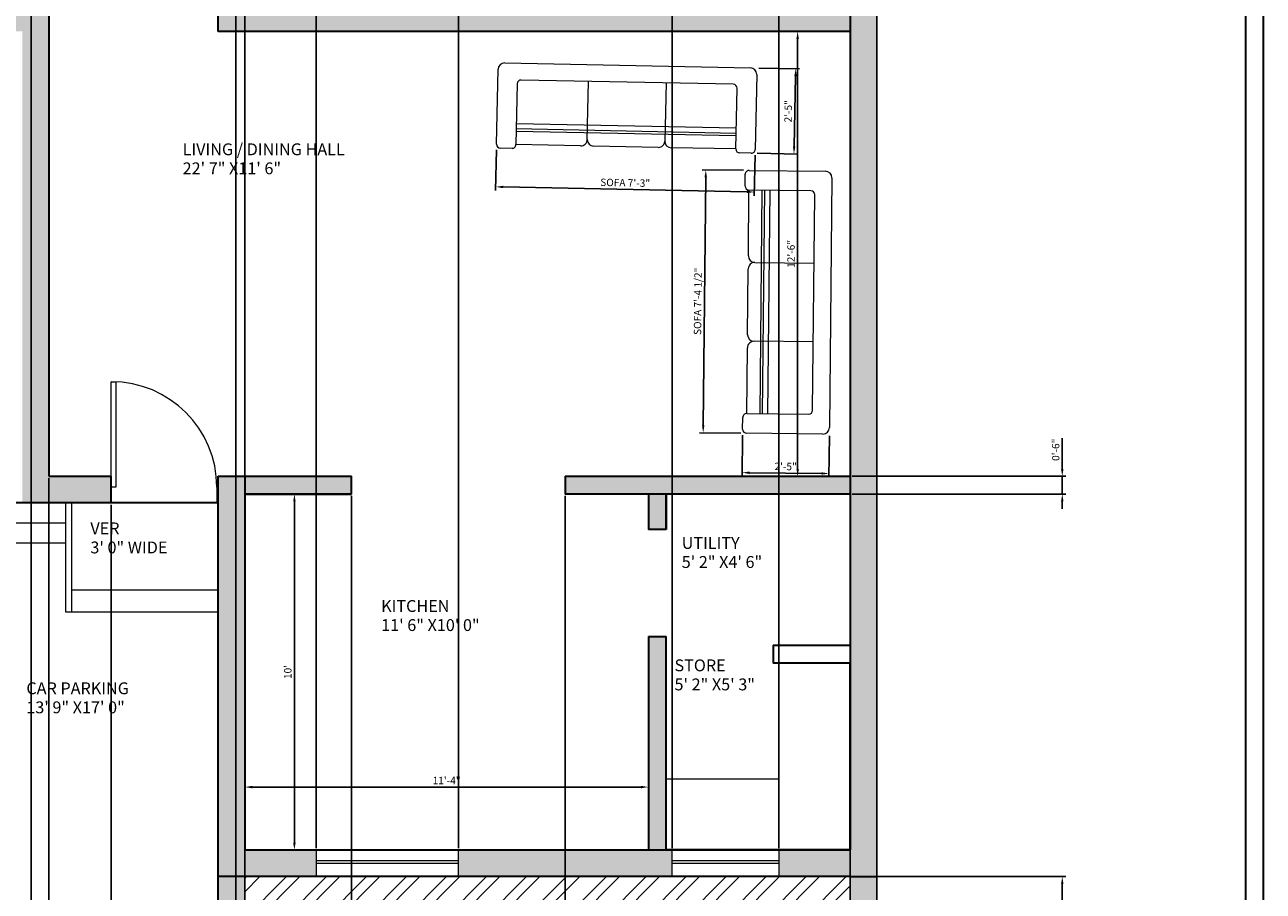
# Model space of a CAD drawing. Units: inches. Extents: x 2004 to 2661, y 1548 to 2351.
# Tile 3 of 5: x 2244 to 2661, y 1748 to 2040. Entities that reach past the tile are written whole.
import ezdxf

# ---------------------------------------------------------------- set-up
doc = ezdxf.new("R2010")
doc.units = ezdxf.units.IN
for name, color, linetype, lineweight in [('A-ANNO-DIMS', 2, 'Continuous', 18), ('A-ANNO-TTLB', 7, 'Continuous', 35), ('A-AREA-IDEN', 7, 'Continuous', 18), ('A-DOOR', 3, 'Continuous', 18), ('A-FLOR-CASE', 8, 'Continuous', 18), ('A-FLOR-STRS', 7, 'Continuous', 18), ('A-FURN', 8, 'Continuous', 18), ('A-GLAZ', 4, 'Continuous', 18), ('A-WALL', 7, 'Continuous', 35), ('C-PROP', 7, 'Continuous', 25)]:
    doc.layers.add(name, color=color, linetype=linetype, lineweight=lineweight)
doc.layers.add('A-FLOR-PATT', color=18, linetype='Continuous', lineweight=13, true_color=0x000000)
doc.layers.add('A-WALL-PATT', color=18, linetype='Continuous', lineweight=13, true_color=0x000000)
doc.styles.get("Standard").update_dxf_attribs({"font": 'arial.ttf'})
doc.dimstyles.new('Copy of ISO-25', dxfattribs={"dimtxt": 2.5, "dimasz": 2.5, "dimexe": 1.25, "dimexo": 0.625, "dimtad": 1, "dimlunit": 4, "dimtxsty": 'Standard', "dimcen": 2.5, "dimadec": 0, "dimazin": 0, "dimtfac": 1, "dimtmove": 0, "dimatfit": 3, "dimfxl": 1, "dimarcsym": 0})

# ---------------------------------------------------------------- blocks, each defined once
blk = doc.blocks.new('A$C05BA3A2B')
for p, q in [((0.05, 0.6596), (1.95, 0.6596)), ((0.05, 0.6596), (1.95, 0.6596)), ((0.05, 0.6596), (1.95, 0.6596)), ((0, 0.03), (0, 0.6096)), ((0, 0.03), (0, 0.6096)), ((0, 0.03), (0, 0.6096)), ((2, 0.6096), (2, 0.03)), ((2, 0.6096), (2, 0.03)), ((2, 0.6096), (2, 0.03)), ((0.15, 0.5), (0.15, 0.03)), ((0.15, 0.5), (0.15, 0.03)), ((0.15, 0.5), (0.15, 0.03)), ((1.82, 0.53), (0.18, 0.53)), ((1.82, 0.53), (0.18, 0.53)), ((1.82, 0.53), (0.18, 0.53)), ((0.7, 0.08), (0.7, 0.53)), ((0.7, 0.08), (0.7, 0.53)), ((0.7, 0.08), (0.7, 0.53)), ((1.3, 0.53), (1.3, 0.08)), ((1.3, 0.53), (1.3, 0.08)), ((1.3, 0.53), (1.3, 0.08)), ((1.85, 0.03), (1.85, 0.5)), ((1.85, 0.03), (1.85, 0.5)), ((1.85, 0.03), (1.85, 0.5)), ((1.85, 0.1908), (0.15, 0.1908)), ((1.85, 0.1908), (0.15, 0.1908)), ((1.85, 0.1908), (0.15, 0.1908)), ((1.85, 0.1508), (0.15, 0.1508)), ((1.85, 0.1508), (0.15, 0.1508)), ((1.85, 0.1508), (0.15, 0.1508)), ((1.85, 0.1308), (0.15, 0.1308)), ((1.85, 0.1308), (0.15, 0.1308)), ((1.85, 0.1308), (0.15, 0.1308)), ((0.12, 0), (0.03, 0)), ((0.12, 0), (0.03, 0)), ((0.12, 0), (0.03, 0)), ((0.65, 0.03), (0.15, 0.03)), ((0.65, 0.03), (0.15, 0.03)), ((0.65, 0.03), (0.15, 0.03)), ((1.25, 0.03), (0.75, 0.03)), ((1.25, 0.03), (0.75, 0.03)), ((1.25, 0.03), (0.75, 0.03)), ((1.85, 0.03), (1.35, 0.03)), ((1.85, 0.03), (1.35, 0.03)), ((1.85, 0.03), (1.35, 0.03)), ((1.97, 0), (1.88, 0)), ((1.97, 0), (1.88, 0)), ((1.97, 0), (1.88, 0))]:
    blk.add_line(p, q)
for centre, radius, start, end in [((0.05, 0.6096), 0.05, 90, 180), ((0.05, 0.6096), 0.05, 90, 180), ((0.05, 0.6096), 0.05, 90, 180), ((1.95, 0.6096), 0.05, 0, 90), ((1.95, 0.6096), 0.05, 0, 90), ((1.95, 0.6096), 0.05, 0, 90), ((0.18, 0.5), 0.03, 90, 180), ((0.18, 0.5), 0.03, 90, 180), ((0.18, 0.5), 0.03, 90, 180), ((1.82, 0.5), 0.03, 0, 90), ((1.82, 0.5), 0.03, 0, 90), ((1.82, 0.5), 0.03, 0, 90), ((0.03, 0.03), 0.03, 180, 270), ((0.03, 0.03), 0.03, 180, 270), ((0.03, 0.03), 0.03, 180, 270), ((0.12, 0.03), 0.03, 270, 0), ((0.12, 0.03), 0.03, 270, 0), ((0.12, 0.03), 0.03, 270, 0), ((0.65, 0.08), 0.05, 270, 0), ((0.65, 0.08), 0.05, 270, 0), ((0.65, 0.08), 0.05, 270, 0), ((0.75, 0.08), 0.05, 180, 270), ((0.75, 0.08), 0.05, 180, 270), ((0.75, 0.08), 0.05, 180, 270), ((1.25, 0.08), 0.05, 270, 0), ((1.25, 0.08), 0.05, 270, 0), ((1.25, 0.08), 0.05, 270, 0), ((1.35, 0.08), 0.05, 180, 270), ((1.35, 0.08), 0.05, 180, 270), ((1.35, 0.08), 0.05, 180, 270), ((1.88, 0.03), 0.03, 180, 270), ((1.88, 0.03), 0.03, 180, 270), ((1.88, 0.03), 0.03, 180, 270), ((1.97, 0.03), 0.03, 270, 0), ((1.97, 0.03), 0.03, 270, 0), ((1.97, 0.03), 0.03, 270, 0)]:
    blk.add_arc(centre, radius, start, end)
blk = doc.blocks.new('*U5')
for p, q in [((0, 0), (0, -6)), ((40, 0), (40, -6))]:
    blk.add_line(p, q)
blk.add_lwpolyline([(0, 0), (0, 40), (1.75, 40), (1.75, 0)], close=True)
blk.add_arc((0, 0), 40, 0, 90)
blk = doc.blocks.new('*D25')
at = {"layer": 'A-ANNO-DIMS', "color": 0, "lineweight": -2, "transparency": 16777216}
for p, q in [((2521.63, 2038.09), (2503.3, 2038.09)), ((2504.55, 2035.59), (2504.55, 1890.59)), ((2521.63, 1888.09), (2503.3, 1888.09))]:
    blk.add_line(p, q, dxfattribs=at)
at = {"layer": 'A-ANNO-DIMS', "color": 0, "transparency": 16777216}
for points in [[(2504.14, 2035.59), (2504.97, 2035.59), (2504.55, 2038.09)], [(2504.14, 1890.59), (2504.97, 1890.59), (2504.55, 1888.09)]]:
    blk.add_solid(points, dxfattribs=at)
at = {"layer": 'Defpoints', "color": 0, "transparency": 16777216}
for p in [(2522.26, 2038.09), (2504.55, 1888.09), (2522.26, 1888.09)]:
    blk.add_point(p, dxfattribs=at)
at = {"layer": 'A-ANNO-DIMS', "color": 0, "transparency": 16777216, "insert": (2502.65, 1963.09), "char_height": 2.5, "attachment_point": 5, "rotation": 90}
blk.add_mtext('12\'-6"', dxfattribs=at)
blk = doc.blocks.new('*D26')
at = {"layer": 'A-ANNO-DIMS', "color": 0, "lineweight": -2, "transparency": 16777216}
for p, q in [((2318.26, 1762.72), (2318.26, 1784.55)), ((2320.76, 1783.3), (2451.76, 1783.3)), ((2454.26, 1762.72), (2454.26, 1784.55))]:
    blk.add_line(p, q, dxfattribs=at)
at = {"layer": 'A-ANNO-DIMS', "color": 0, "transparency": 16777216}
for points in [[(2320.76, 1783.71), (2320.76, 1782.88), (2318.26, 1783.3)], [(2451.76, 1783.71), (2451.76, 1782.88), (2454.26, 1783.3)]]:
    blk.add_solid(points, dxfattribs=at)
at = {"layer": 'Defpoints', "color": 0, "transparency": 16777216}
for p in [(2454.26, 1783.3), (2318.26, 1762.09), (2454.26, 1762.09)]:
    blk.add_point(p, dxfattribs=at)
at = {"layer": 'A-ANNO-DIMS', "color": 0, "transparency": 16777216, "insert": (2386.26, 1785.18), "char_height": 2.5, "attachment_point": 5}
blk.add_mtext('11\'-4"', dxfattribs=at)
blk = doc.blocks.new('*D27')
at = {"layer": 'A-ANNO-DIMS', "color": 0, "lineweight": -2, "transparency": 16777216}
for p, q in [((2318.88, 1882.09), (2336.22, 1882.09)), ((2334.97, 1879.59), (2334.97, 1764.59)), ((2318.88, 1762.09), (2336.22, 1762.09))]:
    blk.add_line(p, q, dxfattribs=at)
at = {"layer": 'A-ANNO-DIMS', "color": 0, "transparency": 16777216}
for points in [[(2334.55, 1879.59), (2335.39, 1879.59), (2334.97, 1882.09)], [(2334.55, 1764.59), (2335.39, 1764.59), (2334.97, 1762.09)]]:
    blk.add_solid(points, dxfattribs=at)
at = {"layer": 'Defpoints', "color": 0, "transparency": 16777216}
for p in [(2318.26, 1882.09), (2318.26, 1762.09), (2334.97, 1762.09)]:
    blk.add_point(p, dxfattribs=at)
at = {"layer": 'A-ANNO-DIMS', "color": 0, "transparency": 16777216, "insert": (2333.07, 1822.09), "char_height": 2.5, "attachment_point": 5, "rotation": 90}
blk.add_mtext("10'", dxfattribs=at)
blk = doc.blocks.new('*D31')
at = {"layer": 'A-ANNO-DIMS', "color": 0, "lineweight": -2, "transparency": 16777216}
for p, q in [((2486.27, 1991.26), (2472.35, 1991.4)), ((2473.57, 1988.89), (2472.73, 1905.24)), ((2485.38, 1902.62), (2471.46, 1902.76))]:
    blk.add_line(p, q, dxfattribs=at)
at = {"layer": 'A-ANNO-DIMS', "color": 0, "transparency": 16777216}
for points in [[(2473.16, 1988.9), (2473.99, 1988.89), (2473.6, 1991.39)], [(2472.32, 1905.25), (2473.15, 1905.24), (2472.71, 1902.74)]]:
    blk.add_solid(points, dxfattribs=at)
at = {"layer": 'Defpoints', "color": 0, "transparency": 16777216}
for p in [(2486.9, 1991.26), (2472.71, 1902.74), (2486, 1902.61)]:
    blk.add_point(p, dxfattribs=at)
at = {"layer": 'A-ANNO-DIMS', "color": 0, "transparency": 16777216, "insert": (2471.23, 1947.09), "char_height": 2.5, "attachment_point": 5, "rotation": 89.4242}
blk.add_mtext('SOFA 7\'-4 1/2"', dxfattribs=at)
blk = doc.blocks.new('*D32')
at = {"layer": 'A-ANNO-DIMS', "color": 0, "lineweight": -2, "transparency": 16777216}
for p, q in [((2486, 1901.99), (2485.86, 1888.06)), ((2515.23, 1901.69), (2515.09, 1887.77)), ((2488.37, 1889.29), (2512.6, 1889.05))]:
    blk.add_line(p, q, dxfattribs=at)
at = {"layer": 'A-ANNO-DIMS', "color": 0, "transparency": 16777216}
for points in [[(2488.37, 1889.71), (2488.37, 1888.87), (2485.87, 1889.31)], [(2512.61, 1889.46), (2512.6, 1888.63), (2515.1, 1889.02)]]:
    blk.add_solid(points, dxfattribs=at)
at = {"layer": 'Defpoints', "color": 0, "transparency": 16777216}
for p in [(2486, 1902.61), (2515.24, 1902.32), (2515.1, 1889.02)]:
    blk.add_point(p, dxfattribs=at)
at = {"layer": 'A-ANNO-DIMS', "color": 0, "transparency": 16777216, "insert": (2500.51, 1891.07), "char_height": 2.5, "attachment_point": 5, "rotation": 359.4242}
blk.add_mtext('2\'-5"', dxfattribs=at)
blk = doc.blocks.new('*D33')
at = {"layer": 'A-ANNO-DIMS', "color": 0, "lineweight": -2, "transparency": 16777216}
for p, q in [((2403.06, 1998.15), (2402.78, 1984.45)), ((2490.22, 1996.4), (2489.95, 1982.7)), ((2405.31, 1985.65), (2487.47, 1984))]:
    blk.add_line(p, q, dxfattribs=at)
at = {"layer": 'A-ANNO-DIMS', "color": 0, "transparency": 16777216}
for points in [[(2405.32, 1986.06), (2405.3, 1985.23), (2402.81, 1985.7)], [(2487.48, 1984.41), (2487.47, 1983.58), (2489.97, 1983.95)]]:
    blk.add_solid(points, dxfattribs=at)
at = {"layer": 'Defpoints', "color": 0, "transparency": 16777216}
for p in [(2403.07, 1998.77), (2490.24, 1997.02), (2489.97, 1983.95)]:
    blk.add_point(p, dxfattribs=at)
at = {"layer": 'A-ANNO-DIMS', "color": 0, "transparency": 16777216, "insert": (2446.43, 1986.74), "char_height": 2.5, "attachment_point": 5, "rotation": 358.8484}
blk.add_mtext('SOFA 7\'-3"', dxfattribs=at)
blk = doc.blocks.new('*D34')
at = {"layer": 'A-ANNO-DIMS', "color": 0, "lineweight": -2, "transparency": 16777216}
for p, q in [((2491.44, 2025.75), (2505.14, 2025.48)), ((2503.36, 1999.26), (2503.84, 2023)), ((2490.86, 1997.01), (2504.56, 1996.73))]:
    blk.add_line(p, q, dxfattribs=at)
at = {"layer": 'A-ANNO-DIMS', "color": 0, "transparency": 16777216}
for points in [[(2503.42, 2023.01), (2504.26, 2023), (2503.89, 2025.5)], [(2502.95, 1999.27), (2503.78, 1999.25), (2503.31, 1996.76)]]:
    blk.add_solid(points, dxfattribs=at)
at = {"layer": 'Defpoints', "color": 0, "transparency": 16777216}
for p in [(2490.81, 2025.77), (2503.89, 2025.5), (2490.24, 1997.02)]:
    blk.add_point(p, dxfattribs=at)
at = {"layer": 'A-ANNO-DIMS', "color": 0, "transparency": 16777216, "insert": (2501.7, 2011.17), "char_height": 2.5, "attachment_point": 5, "rotation": 88.8484}
blk.add_mtext('2\'-5"', dxfattribs=at)
blk = doc.blocks.new('*D37')
at = {"layer": 'A-ANNO-DIMS', "color": 0, "lineweight": -2, "transparency": 16777216}
for p, q in [((2246.26, 2082.47), (2246.26, 1630.09)), ((2144.26, 2046.47), (2144.26, 1630.09)), ((2146.76, 1631.34), (2243.76, 1631.34))]:
    blk.add_line(p, q, dxfattribs=at)
at = {"layer": 'A-ANNO-DIMS', "color": 0, "transparency": 16777216}
for points in [[(2146.76, 1631.76), (2146.76, 1630.93), (2144.26, 1631.34)], [(2243.76, 1631.76), (2243.76, 1630.93), (2246.26, 1631.34)]]:
    blk.add_solid(points, dxfattribs=at)
at = {"layer": 'Defpoints', "color": 0, "transparency": 16777216}
for p in [(2246.26, 2083.09), (2144.26, 2047.09), (2246.26, 1631.34)]:
    blk.add_point(p, dxfattribs=at)
at = {"layer": 'A-ANNO-DIMS', "color": 0, "transparency": 16777216, "insert": (2195.26, 1633.24), "char_height": 2.5, "attachment_point": 5}
blk.add_mtext('8\'-6"', dxfattribs=at)
blk = doc.blocks.new('*D39')
at = {"layer": 'A-ANNO-DIMS', "color": 0, "lineweight": -2, "transparency": 16777216}
for p, q in [((2252.26, 1887.47), (2252.26, 1630.09)), ((2522.26, 1887.47), (2522.26, 1630.09)), ((2254.76, 1631.34), (2519.76, 1631.34))]:
    blk.add_line(p, q, dxfattribs=at)
at = {"layer": 'A-ANNO-DIMS', "color": 0, "transparency": 16777216}
for points in [[(2254.76, 1631.76), (2254.76, 1630.93), (2252.26, 1631.34)], [(2519.76, 1631.76), (2519.76, 1630.93), (2522.26, 1631.34)]]:
    blk.add_solid(points, dxfattribs=at)
at = {"layer": 'Defpoints', "color": 0, "transparency": 16777216}
for p in [(2252.26, 1888.09), (2522.26, 1888.09), (2522.26, 1631.34)]:
    blk.add_point(p, dxfattribs=at)
at = {"layer": 'A-ANNO-DIMS', "color": 0, "transparency": 16777216, "insert": (2387.26, 1633.24), "char_height": 2.5, "attachment_point": 5}
blk.add_mtext('22\'-6"', dxfattribs=at)
blk = doc.blocks.new('*D40')
at = {"layer": 'A-ANNO-DIMS', "color": 0, "lineweight": -2, "transparency": 16777216}
for p, q in [((2522.88, 1753.09), (2594.98, 1753.09)), ((2593.73, 1750.59), (2593.73, 1677.59)), ((2522.88, 1675.09), (2594.98, 1675.09))]:
    blk.add_line(p, q, dxfattribs=at)
at = {"layer": 'A-ANNO-DIMS', "color": 0, "transparency": 16777216}
for points in [[(2593.31, 1750.59), (2594.15, 1750.59), (2593.73, 1753.09)], [(2593.31, 1677.59), (2594.15, 1677.59), (2593.73, 1675.09)]]:
    blk.add_solid(points, dxfattribs=at)
at = {"layer": 'Defpoints', "color": 0, "transparency": 16777216}
for p in [(2522.26, 1753.09), (2522.26, 1675.09), (2593.73, 1675.09)]:
    blk.add_point(p, dxfattribs=at)
at = {"layer": 'A-ANNO-DIMS', "color": 0, "transparency": 16777216, "insert": (2591.83, 1714.09), "char_height": 2.5, "attachment_point": 5, "rotation": 90}
blk.add_mtext('6\'-6"', dxfattribs=at)
blk = doc.blocks.new('*D41')
at = {"layer": 'A-ANNO-DIMS', "color": 0, "lineweight": -2, "transparency": 16777216}
for p, q in [((2318.26, 1675.72), (2318.26, 2346.91)), ((2320.76, 2345.66), (2519.76, 2345.66)), ((2522.26, 1675.72), (2522.26, 2346.91))]:
    blk.add_line(p, q, dxfattribs=at)
at = {"layer": 'A-ANNO-DIMS', "color": 0, "transparency": 16777216}
for points in [[(2320.76, 2346.07), (2320.76, 2345.24), (2318.26, 2345.66)], [(2519.76, 2346.07), (2519.76, 2345.24), (2522.26, 2345.66)]]:
    blk.add_solid(points, dxfattribs=at)
at = {"layer": 'Defpoints', "color": 0, "transparency": 16777216}
for p in [(2522.26, 2345.66), (2318.26, 1675.09), (2522.26, 1675.09)]:
    blk.add_point(p, dxfattribs=at)
at = {"layer": 'A-ANNO-DIMS', "color": 0, "transparency": 16777216, "insert": (2420.26, 2347.56), "char_height": 2.5, "attachment_point": 5}
blk.add_mtext('17\'-0"', dxfattribs=at)
blk = doc.blocks.new('*D42')
at = {"layer": 'A-ANNO-DIMS', "color": 0, "lineweight": -2, "transparency": 16777216}
for p, q in [((2315.26, 2256.47), (2315.26, 1630.09)), ((2522.26, 2256.47), (2522.26, 1630.09)), ((2317.76, 1631.34), (2519.76, 1631.34))]:
    blk.add_line(p, q, dxfattribs=at)
at = {"layer": 'A-ANNO-DIMS', "color": 0, "transparency": 16777216}
for points in [[(2317.76, 1631.76), (2317.76, 1630.93), (2315.26, 1631.34)], [(2519.76, 1631.76), (2519.76, 1630.93), (2522.26, 1631.34)]]:
    blk.add_solid(points, dxfattribs=at)
at = {"layer": 'Defpoints', "color": 0, "transparency": 16777216}
for p in [(2315.26, 2257.09), (2522.26, 2257.09), (2522.26, 1631.34)]:
    blk.add_point(p, dxfattribs=at)
at = {"layer": 'A-ANNO-DIMS', "color": 0, "transparency": 16777216, "insert": (2418.76, 1633.24), "char_height": 2.5, "attachment_point": 5}
blk.add_mtext('17\'-3"', dxfattribs=at)
blk = doc.blocks.new('*D44')
at = {"layer": 'A-ANNO-DIMS', "color": 0, "lineweight": -2, "transparency": 16777216}
for p, q in [((2593.73, 1890.59), (2593.73, 1900.99)), ((2522.88, 1888.09), (2594.98, 1888.09)), ((2593.73, 1882.09), (2593.73, 1888.09)), ((2522.88, 1882.09), (2594.98, 1882.09)), ((2593.73, 1879.59), (2593.73, 1877.09))]:
    blk.add_line(p, q, dxfattribs=at)
at = {"layer": 'A-ANNO-DIMS', "color": 0, "transparency": 16777216}
for points in [[(2593.31, 1890.59), (2594.15, 1890.59), (2593.73, 1888.09)], [(2593.31, 1879.59), (2594.15, 1879.59), (2593.73, 1882.09)]]:
    blk.add_solid(points, dxfattribs=at)
at = {"layer": 'Defpoints', "color": 0, "transparency": 16777216}
for p in [(2522.26, 1888.09), (2593.73, 1888.09), (2522.26, 1882.09)]:
    blk.add_point(p, dxfattribs=at)
at = {"layer": 'A-ANNO-DIMS', "color": 0, "transparency": 16777216, "insert": (2591.83, 1897.04), "char_height": 2.5, "attachment_point": 5, "rotation": 90}
blk.add_mtext('0\'-6"', dxfattribs=at)
blk = doc.blocks.new('*D45')
at = {"layer": 'A-ANNO-DIMS', "color": 0, "lineweight": -2, "transparency": 16777216}
for p, q in [((2273.26, 1878.47), (2273.26, 1630.09)), ((2309.26, 1878.47), (2309.26, 1630.09)), ((2275.76, 1631.34), (2306.76, 1631.34))]:
    blk.add_line(p, q, dxfattribs=at)
at = {"layer": 'A-ANNO-DIMS', "color": 0, "transparency": 16777216}
for points in [[(2275.76, 1631.76), (2275.76, 1630.93), (2273.26, 1631.34)], [(2306.76, 1631.76), (2306.76, 1630.93), (2309.26, 1631.34)]]:
    blk.add_solid(points, dxfattribs=at)
at = {"layer": 'Defpoints', "color": 0, "transparency": 16777216}
for p in [(2273.26, 1879.09), (2309.26, 1879.09), (2309.26, 1631.34)]:
    blk.add_point(p, dxfattribs=at)
at = {"layer": 'A-ANNO-DIMS', "color": 0, "transparency": 16777216, "insert": (2291.26, 1633.24), "char_height": 2.5, "attachment_point": 5}
blk.add_mtext('3\'-0"', dxfattribs=at)
blk = doc.blocks.new('*D47')
at = {"layer": 'A-ANNO-DIMS', "color": 0, "lineweight": -2, "transparency": 16777216}
for p, q in [((2354.26, 1881.47), (2354.26, 1630.09)), ((2426.26, 1881.47), (2426.26, 1630.09)), ((2356.76, 1631.34), (2423.76, 1631.34))]:
    blk.add_line(p, q, dxfattribs=at)
at = {"layer": 'A-ANNO-DIMS', "color": 0, "transparency": 16777216}
for points in [[(2356.76, 1631.76), (2356.76, 1630.93), (2354.26, 1631.34)], [(2423.76, 1631.76), (2423.76, 1630.93), (2426.26, 1631.34)]]:
    blk.add_solid(points, dxfattribs=at)
at = {"layer": 'Defpoints', "color": 0, "transparency": 16777216}
for p in [(2354.26, 1882.09), (2426.26, 1882.09), (2426.26, 1631.34)]:
    blk.add_point(p, dxfattribs=at)
at = {"layer": 'A-ANNO-DIMS', "color": 0, "transparency": 16777216, "insert": (2390.26, 1633.24), "char_height": 2.5, "attachment_point": 5}
blk.add_mtext('6\'-0"', dxfattribs=at)
blk = doc.blocks.new('*D50')
at = {"layer": 'A-ANNO-DIMS', "color": 0, "lineweight": -2, "transparency": 16777216}
for p, q in [((2318.26, 1762.72), (2318.26, 2346.91)), ((2320.76, 2345.66), (2339.76, 2345.66)), ((2342.26, 1762.72), (2342.26, 2346.91))]:
    blk.add_line(p, q, dxfattribs=at)
at = {"layer": 'A-ANNO-DIMS', "color": 0, "transparency": 16777216}
for points in [[(2320.76, 2346.07), (2320.76, 2345.24), (2318.26, 2345.66)], [(2339.76, 2346.07), (2339.76, 2345.24), (2342.26, 2345.66)]]:
    blk.add_solid(points, dxfattribs=at)
at = {"layer": 'Defpoints', "color": 0, "transparency": 16777216}
for p in [(2342.26, 2345.66), (2318.26, 1762.09), (2342.26, 1762.09)]:
    blk.add_point(p, dxfattribs=at)
at = {"layer": 'A-ANNO-DIMS', "color": 0, "transparency": 16777216, "insert": (2330.26, 2347.56), "char_height": 2.5, "attachment_point": 5}
blk.add_mtext('2\'-0"', dxfattribs=at)
blk = doc.blocks.new('*D51')
at = {"layer": 'A-ANNO-DIMS', "color": 0, "lineweight": -2, "transparency": 16777216}
for p, q in [((2342.26, 1762.72), (2342.26, 2346.91)), ((2344.76, 2345.66), (2387.76, 2345.66)), ((2390.26, 1762.72), (2390.26, 2346.91))]:
    blk.add_line(p, q, dxfattribs=at)
at = {"layer": 'A-ANNO-DIMS', "color": 0, "transparency": 16777216}
for points in [[(2344.76, 2346.07), (2344.76, 2345.24), (2342.26, 2345.66)], [(2387.76, 2346.07), (2387.76, 2345.24), (2390.26, 2345.66)]]:
    blk.add_solid(points, dxfattribs=at)
at = {"layer": 'Defpoints', "color": 0, "transparency": 16777216}
for p in [(2390.26, 2345.66), (2342.26, 1762.09), (2390.26, 1762.09)]:
    blk.add_point(p, dxfattribs=at)
at = {"layer": 'A-ANNO-DIMS', "color": 0, "transparency": 16777216, "insert": (2366.26, 2347.56), "char_height": 2.5, "attachment_point": 5}
blk.add_mtext('4\'-0"', dxfattribs=at)
blk = doc.blocks.new('*D52')
at = {"layer": 'A-ANNO-DIMS', "color": 0, "lineweight": -2, "transparency": 16777216}
for p, q in [((2462.26, 1762.72), (2462.26, 2346.91)), ((2464.76, 2345.66), (2495.76, 2345.66)), ((2498.26, 1762.72), (2498.26, 2346.91))]:
    blk.add_line(p, q, dxfattribs=at)
at = {"layer": 'A-ANNO-DIMS', "color": 0, "transparency": 16777216}
for points in [[(2464.76, 2346.07), (2464.76, 2345.24), (2462.26, 2345.66)], [(2495.76, 2346.07), (2495.76, 2345.24), (2498.26, 2345.66)]]:
    blk.add_solid(points, dxfattribs=at)
at = {"layer": 'Defpoints', "color": 0, "transparency": 16777216}
for p in [(2498.26, 2345.66), (2462.26, 1762.09), (2498.26, 1762.09)]:
    blk.add_point(p, dxfattribs=at)
at = {"layer": 'A-ANNO-DIMS', "color": 0, "transparency": 16777216, "insert": (2480.26, 2347.56), "char_height": 2.5, "attachment_point": 5}
blk.add_mtext('3\'-0"', dxfattribs=at)
blk = doc.blocks.new('*D53')
at = {"layer": 'A-ANNO-DIMS', "color": 0, "lineweight": -2, "transparency": 16777216}
for p, q in [((2498.26, 1762.72), (2498.26, 2346.91)), ((2500.76, 2345.66), (2519.76, 2345.66)), ((2522.26, 1762.72), (2522.26, 2346.91))]:
    blk.add_line(p, q, dxfattribs=at)
at = {"layer": 'A-ANNO-DIMS', "color": 0, "transparency": 16777216}
for points in [[(2500.76, 2346.07), (2500.76, 2345.24), (2498.26, 2345.66)], [(2519.76, 2346.07), (2519.76, 2345.24), (2522.26, 2345.66)]]:
    blk.add_solid(points, dxfattribs=at)
at = {"layer": 'Defpoints', "color": 0, "transparency": 16777216}
for p in [(2522.26, 2345.66), (2498.26, 1762.09), (2522.26, 1762.09)]:
    blk.add_point(p, dxfattribs=at)
at = {"layer": 'A-ANNO-DIMS', "color": 0, "transparency": 16777216, "insert": (2510.26, 2347.56), "char_height": 2.5, "attachment_point": 5}
blk.add_mtext('2\'-0"', dxfattribs=at)

msp = doc.modelspace()

# ---------------------------------------------------------------- hatches: boundary and pattern name
at = {"layer": 'A-FLOR-PATT'}
h = msp.add_hatch(dxfattribs=at)
h.set_pattern_fill('ANSI32', color=256)
h.paths.add_polyline_path([(2522.257, 2257.093), (2466.833, 2257.093), (2315.257, 2257.093), (2418.757, 2233.093)])
h.paths.add_polyline_path([(2418.757, 2233.093), (2315.257, 2257.093), (2315.257, 2209.093)])
h.paths.add_polyline_path([(2418.757, 2233.093), (2315.257, 2209.093), (2522.257, 2209.093)])
h.paths.add_polyline_path([(2522.257, 2257.093), (2418.757, 2233.093), (2522.257, 2209.093)])
h.paths.add_polyline_path([(2522.257, 1753.093), (2318.257, 1753.093), (2318.257, 1675.093), (2522.257, 1675.093)])
h.paths.add_polyline_path([(2210.267, 2081.517), (2210.233, 2081.517), (2210.233, 2083.093), (2246.257, 2083.093), (2246.257, 2119.093), (2144.257, 2119.093), (2144.257, 2047.093), (2244.938, 2047.093, -0.390864)])
h.paths.add_polyline_path([(2171.613, 2077.721), (2161.069, 2080.96), (2161.193, 2075.729), (2163.808, 2075.791), (2163.932, 2070.56), (2162.189, 2070.519), (2162.106, 2074.006), (2161.234, 2073.986), (2161.338, 2069.627), (2147.389, 2069.296), (2146.521, 2105.911), (2160.469, 2106.241), (2160.738, 2094.908), (2171.117, 2098.643, -0.7025712), (2195.775, 2088.761, -0.7025621)], flags=16)
h.paths.add_polyline_path([(2171.53, 2081.208), (2171.2, 2095.156, -0.7345333), (2194.031, 2088.72, -0.7345297)], flags=0)
h.paths.add_polyline_path([(2158.245, 2071.298), (2150.835, 2071.122, -0.4142136), (2149.061, 2072.388), (2148.347, 2102.465, -0.4142136), (2149.614, 2104.239), (2157.024, 2104.415, -0.4142136), (2158.798, 2103.149), (2159.512, 2073.072, -0.4142136)], flags=0)
h.paths.add_polyline_path([(2522.257, 2200.093), (2517.397, 2200.093), (2517.397, 2185.232), (2505.384, 2185.232), (2509.08, 2174.143, -0.7025712), (2497.991, 2148.268, -0.7025621), (2486.902, 2174.142), (2490.599, 2185.232), (2485.054, 2185.232), (2485.054, 2182.459), (2479.509, 2182.459), (2479.509, 2184.307), (2483.206, 2184.307), (2483.206, 2185.232), (2478.585, 2185.232), (2478.585, 2200.093), (2459.257, 2200.093), (2459.257, 2106.686, -0.3761573), (2493.676, 2139.619), (2493.676, 2139.653), (2495.257, 2139.653), (2495.257, 2104.093), (2522.257, 2104.093)])
h.paths.add_polyline_path([(2349.854, 1719.146), (2381.921, 1719.146), (2381.921, 1725.273), (2349.854, 1725.273)], flags=24)
h.paths.add_polyline_path([(2349.84, 1725.558), (2388.851, 1725.558), (2388.851, 1731.767), (2349.84, 1731.767)], flags=24)
h.paths.add_polyline_path([(2152.908, 2086.679), (2181.867, 2086.679), (2181.867, 2092.806), (2152.908, 2092.806)], flags=8)
h.paths.add_polyline_path([(2152.895, 2093.091), (2174.525, 2093.091), (2174.525, 2099.3), (2152.895, 2099.3)], flags=8)
h.paths.add_polyline_path([(2515.001, 2150.174), (2515.001, 2154.033), (2509.85, 2154.033), (2509.85, 2150.174)], flags=24)
h.paths.add_polyline_path([(2469.272, 2171.563), (2498.231, 2171.563), (2498.231, 2177.69), (2469.272, 2177.69)], flags=24)
h.paths.add_polyline_path([(2469.258, 2177.975), (2490.888, 2177.975), (2490.888, 2184.184), (2469.258, 2184.184)], flags=24)
at = {"layer": 'A-WALL-PATT'}
h = msp.add_hatch(color=256, dxfattribs=at)
h.dxf.hatch_style = 1
h.paths.add_polyline_path([(2315.257, 2266.093), (2135.257, 2266.093), (2135.257, 1666.093), (2531.257, 1666.093), (2531.257, 1753.093), (2522.257, 1753.093), (2522.257, 1675.093), (2144.257, 1675.093), (2144.257, 2038.093), (2180.257, 2038.093), (2180.257, 2047.093), (2144.257, 2047.093), (2144.257, 2257.093), (2309.257, 2257.093), (2315.257, 2257.093)])
h.paths.add_polyline_path([(2522.257, 2266.093), (2315.257, 2266.093), (2315.257, 2257.093), (2522.257, 2257.093)], flags=17)
h.paths.add_polyline_path([(2368.773, 2209.093), (2315.257, 2209.093), (2309.257, 2209.093), (2309.257, 2119.093), (2309.257, 2083.093), (2315.257, 2083.093), (2315.257, 2119.093), (2315.257, 2200.093), (2368.773, 2200.093)], flags=17)
h.paths.add_polyline_path([(2459.257, 2209.093), (2428.773, 2209.093), (2428.773, 2200.093), (2453.257, 2200.093), (2459.257, 2200.093)], flags=17)
h.paths.add_polyline_path([(2522.257, 2209.093), (2483.257, 2209.093), (2483.257, 2200.093), (2522.257, 2200.093)], flags=17)
h.paths.add_polyline_path([(2522.257, 2044.093), (2459.257, 2044.093), (2459.257, 2056.073, -0.004139), (2458.66, 2056.069), (2453.257, 2056.069), (2453.257, 2044.093), (2315.257, 2044.093), (2315.257, 2046.941, -0.0039864), (2314.68, 2046.936), (2309.257, 2046.936), (2309.257, 2038.093), (2315.257, 2038.093), (2522.257, 2038.093)], flags=17)
h.paths.add_polyline_path([(2531.257, 2266.093), (2522.257, 2266.093), (2522.257, 2257.093), (2522.257, 2209.093), (2522.257, 2200.093), (2522.257, 2104.093), (2522.257, 1762.093), (2498.257, 1762.093), (2498.257, 1753.093), (2522.257, 1753.093), (2531.257, 1753.093)], flags=17)
h.paths.add_polyline_path([(2522.257, 2104.093), (2495.257, 2104.093), (2495.257, 2103.514), (2495.257, 2098.093), (2503.401, 2098.093), (2522.257, 2098.093)], flags=17)
h.paths.add_polyline_path([(2455.748, 2073.874), (2484.708, 2073.874), (2484.708, 2080.001), (2455.748, 2080.001)], flags=25)
h.paths.add_polyline_path([(2455.735, 2080.287), (2477.056, 2080.287), (2477.056, 2086.492), (2455.735, 2086.492)], flags=25)
h.paths.add_polyline_path([(2469.272, 2171.563), (2498.231, 2171.563), (2498.231, 2177.69), (2469.272, 2177.69)], flags=25)
h.paths.add_polyline_path([(2469.258, 2177.975), (2490.888, 2177.975), (2490.888, 2184.184), (2469.258, 2184.184)], flags=25)
h.paths.add_polyline_path([(2360.849, 2078.511), (2396.023, 2078.511), (2396.023, 2084.638), (2360.849, 2084.638)], flags=25)
h.paths.add_polyline_path([(2360.835, 2084.923), (2394.883, 2084.923), (2394.883, 2091.132), (2360.835, 2091.132)], flags=25)
h = msp.add_hatch(color=256, dxfattribs=at)
h.dxf.hatch_style = 1
h.paths.add_polyline_path([(2252.257, 2038.093), (2252.257, 2047.093), (2246.257, 2047.093), (2204.257, 2047.093), (2204.257, 2038.093), (2243.257, 2038.093), (2243.257, 1888.093), (2243.257, 1879.093), (2273.257, 1879.093), (2273.257, 1888.093), (2252.257, 1888.093)])
h.paths.add_polyline_path([(2273.257, 2125.093), (2144.257, 2125.093), (2144.257, 2119.093), (2246.257, 2119.093), (2273.257, 2119.093)])
h.paths.add_polyline_path([(2459.257, 2200.093), (2453.257, 2200.093), (2453.257, 2092.093), (2459.257, 2092.093)])
h.paths.add_polyline_path([(2522.257, 1888.093), (2426.257, 1888.093), (2426.257, 1882.093), (2522.257, 1882.093)])
h.paths.add_polyline_path([(2460.257, 1834.093), (2454.257, 1834.093), (2454.257, 1762.093), (2460.257, 1762.093)])
h.paths.add_polyline_path([(2460.257, 1882.093), (2454.257, 1882.093), (2454.257, 1870.093), (2460.257, 1870.093)])
h.paths.add_polyline_path([(2462.257, 1762.093), (2460.257, 1762.093), (2454.257, 1762.093), (2390.257, 1762.093), (2390.257, 1753.093), (2462.257, 1753.093)])
h.paths.add_polyline_path([(2342.257, 1762.093), (2318.257, 1762.093), (2318.257, 1882.093), (2318.257, 1888.093), (2309.257, 1888.093), (2309.257, 1879.093), (2309.257, 1753.093), (2318.257, 1753.093), (2342.257, 1753.093)])
h.paths.add_polyline_path([(2354.257, 1888.093), (2318.257, 1888.093), (2318.257, 1882.093), (2354.257, 1882.093)])
h.paths.add_polyline_path([(2318.257, 1753.093), (2309.257, 1753.093), (2309.257, 1675.093), (2318.257, 1675.093)])
h.paths.add_polyline_path([(2207.257, 1884.43), (2207.257, 1888.093), (2183.257, 1888.093), (2183.257, 1879.093), (2207.257, 1879.093)])
h.paths.add_polyline_path([(2252.257, 2119.093), (2246.257, 2119.093), (2246.257, 2083.093), (2251.66, 2083.093), (2252.257, 2083.093)])
h.paths.add_polyline_path([(2315.257, 2257.093), (2309.257, 2257.093), (2309.257, 2209.093), (2315.257, 2209.093)])

# ---------------------------------------------------------------- linework, layer by layer
at = {"layer": 'A-ANNO-TTLB'}
for points in [[(2014.058, 2344.754), (2661.447, 2344.754), (2661.447, 1548.19), (2014.058, 1548.19)], [(2020.058, 2338.754), (2655.447, 2338.754), (2655.447, 1554.19), (2020.058, 1554.19)]]:
    msp.add_lwpolyline(points, close=True, dxfattribs=at)
at = {"layer": 'A-FLOR-CASE'}
for p, q in [((2522.257, 1882.093), (2498.257, 1882.093)), ((2498.257, 1882.093), (2498.257, 1831.093)), ((2498.257, 1825.093), (2498.257, 1786.093)), ((2460.257, 1762.093), (2460.257, 1786.093)), ((2460.257, 1786.093), (2498.257, 1786.093))]:
    msp.add_line(p, q, dxfattribs=at)
at = {"layer": 'A-FLOR-STRS'}
for p, q in [((2309.257, 1879.093), (2257.874, 1879.093)), ((2257.874, 1879.093), (2257.874, 1842.347)), ((2257.874, 1879.093), (2259.874, 1879.093)), ((2259.874, 1879.093), (2259.874, 1842.347)), ((2186.568, 1872.355), (2257.874, 1872.355)), ((2186.568, 1865.618), (2257.874, 1865.618)), ((2259.874, 1849.765), (2309.257, 1849.765)), ((2257.874, 1842.347), (2309.257, 1842.347)), ((2309.257, 1842.347), (2309.257, 1842.347))]:
    msp.add_line(p, q, dxfattribs=at)
at = {"layer": 'A-GLAZ'}
for p, q in [((2342.257, 1762.093), (2342.257, 1753.093)), ((2390.257, 1753.093), (2390.257, 1762.093)), ((2462.257, 1753.093), (2462.257, 1762.093)), ((2498.257, 1762.093), (2498.257, 1753.093)), ((2342.257, 1758.593), (2390.257, 1758.593)), ((2342.257, 1757.593), (2390.257, 1757.593)), ((2462.257, 1758.593), (2498.257, 1758.593)), ((2462.257, 1757.593), (2498.257, 1757.593)), ((2342.257, 1753.093), (2378.257, 1753.093)), ((2378.257, 1753.093), (2390.257, 1753.093)), ((2498.257, 1753.093), (2462.257, 1753.093))]:
    msp.add_line(p, q, dxfattribs=at)
at = {"layer": 'A-WALL'}
for p, q in [((2522.257, 2257.093), (2522.257, 1762.093)), ((2252.257, 2047.093), (2252.257, 2038.093)), ((2309.257, 2038.093), (2309.257, 2047.093)), ((2522.257, 2044.093), (2522.257, 2038.093)), ((2252.257, 2038.093), (2252.257, 1888.093)), ((2315.257, 2038.093), (2309.257, 2038.093)), ((2522.257, 2038.093), (2315.257, 2038.093)), ((2252.257, 1888.093), (2273.257, 1888.093)), ((2273.257, 1879.093), (2273.257, 1888.093)), ((2309.257, 1888.093), (2318.257, 1888.093)), ((2309.257, 1879.093), (2309.257, 1888.093)), ((2318.257, 1888.093), (2318.257, 1762.093)), ((2318.257, 1888.093), (2354.257, 1888.093)), ((2354.257, 1882.093), (2354.257, 1888.093)), ((2426.257, 1888.093), (2426.257, 1882.093)), ((2426.257, 1888.093), (2522.257, 1888.093)), ((2522.257, 1888.093), (2522.257, 1882.093)), ((2309.257, 1879.093), (2144.257, 1879.093)), ((2309.257, 1879.093), (2273.257, 1879.093)), ((2309.257, 1675.093), (2309.257, 1879.093)), ((2318.257, 1882.093), (2318.257, 1762.093)), ((2318.257, 1882.093), (2354.257, 1882.093)), ((2354.257, 1882.093), (2318.257, 1882.093)), ((2522.257, 1882.093), (2426.257, 1882.093)), ((2460.257, 1882.093), (2454.257, 1882.093)), ((2454.257, 1882.093), (2454.257, 1870.093)), ((2460.257, 1882.093), (2460.257, 1870.093)), ((2460.257, 1870.093), (2460.257, 1882.093)), ((2460.257, 1870.093), (2454.257, 1870.093)), ((2454.257, 1834.093), (2460.257, 1834.093)), ((2454.257, 1834.093), (2454.257, 1762.093)), ((2460.257, 1762.093), (2460.257, 1834.093)), ((2460.257, 1825.093), (2460.257, 1831.093)), ((2496.257, 1831.093), (2522.257, 1831.093)), ((2496.257, 1831.093), (2496.257, 1825.093)), ((2522.257, 1825.093), (2496.257, 1825.093)), ((2522.257, 1762.093), (2522.257, 1825.093)), ((2318.257, 1762.093), (2522.257, 1762.093)), ((2318.257, 1762.093), (2342.257, 1762.093)), ((2522.257, 1762.093), (2460.257, 1762.093)), ((2522.257, 1762.093), (2498.257, 1762.093)), ((2318.257, 1753.093), (2309.257, 1753.093)), ((2522.257, 1753.093), (2318.257, 1753.093)), ((2522.257, 1753.093), (2531.257, 1753.093))]:
    msp.add_line(p, q, dxfattribs=at)
at = {"layer": 'C-PROP'}
for p, q in [((2531.257, 2266.093), (2531.257, 1666.093)), ((2318.257, 1753.093), (2318.257, 1675.093)), ((2522.257, 1753.093), (2522.257, 1675.093))]:
    msp.add_line(p, q, dxfattribs=at)

# ---------------------------------------------------------------- block references
at = {"layer": 'A-DOOR', "xscale": 0.8891050772908728, "yscale": 0.8891050772908728, "zscale": 0.8891050772908728}
msp.add_blockref('*U5', (2273.257, 1884.427), dxfattribs=at)
at = {"layer": 'A-FURN'}
for p, xscale, yscale, zscale, rotation in [((2403.071, 1998.773), 43.59201171863692, 43.59201171863692, 43.59201171863692, 358.8484214216911), ((2486.895, 1991.258), 44.32570863293522, 44.32570863293522, 44.32570863293522, 269.4242107108455)]:
    msp.add_blockref('A$C05BA3A2B', p, dxfattribs=dict(at, xscale=xscale, yscale=yscale, zscale=zscale, rotation=rotation))

# ---------------------------------------------------------------- texts
at = {"layer": 'A-AREA-IDEN'}
for s, p in [('LIVING / DINING HALL', (2297.304, 1996.349)), ('22\' 7" X11\' 6"', (2297.304, 1989.923)), ('VER', (2266.215, 1868.522)), ('3\' 0" WIDE', (2266.215, 1862.097)), ('UTILITY', (2465.486, 1863.614)), ('5\' 2" X4\' 6"', (2465.486, 1857.188)), ('KITCHEN', (2364.211, 1842.347)), ('11\' 6" X10\' 0"', (2364.211, 1835.922)), ('STORE', (2463.057, 1822.335)), ('5\' 2" X5\' 3"', (2463.057, 1815.91)), ('CAR PARKING', (2244.633, 1814.603)), ('13\' 9" X17\' 0"', (2244.633, 1808.178))]:
    msp.add_text(s, height=4, dxfattribs=at).set_placement(p)

# ---------------------------------------------------------------- dimensions: what is measured, and where the dimension line sits
at = {"layer": 'A-ANNO-DIMS'}
for base, p1, p2, override, picture, middle in [((2522.257, 2345.658), (2318.257, 1675.093), (2522.257, 1675.093), {"dimdec": 1, "dimlfac": 1, "dimrnd": 0, "dimzin": 1, "dimdsep": 46, "dimlunit": 4, "dimfrac": 2}, '*D41', (2420.257, 2347.559)), ((2342.257, 2345.658), (2318.257, 1762.093), (2342.257, 1762.093), {"dimdec": 1, "dimlfac": 1, "dimrnd": 0, "dimzin": 1, "dimdsep": 46, "dimlunit": 4, "dimfrac": 2}, '*D50', (2330.257, 2347.559)), ((2390.257, 2345.658), (2342.257, 1762.093), (2390.257, 1762.093), {"dimdec": 1, "dimlfac": 1, "dimrnd": 0, "dimzin": 1, "dimdsep": 46, "dimlunit": 4, "dimfrac": 2}, '*D51', (2366.257, 2347.559)), ((2498.257, 2345.658), (2462.257, 1762.093), (2498.257, 1762.093), {"dimdec": 1, "dimlfac": 1, "dimrnd": 0, "dimzin": 1, "dimdsep": 46, "dimlunit": 4, "dimfrac": 2}, '*D52', (2480.257, 2347.56)), ((2522.257, 2345.658), (2498.257, 1762.093), (2522.257, 1762.093), {"dimdec": 1, "dimlfac": 1, "dimrnd": 0, "dimzin": 1, "dimdsep": 46, "dimlunit": 4, "dimfrac": 2}, '*D53', (2510.257, 2347.559)), ((2522.257, 1631.343), (2315.257, 2257.093), (2522.257, 2257.093), {"dimdec": 1, "dimlfac": 1, "dimrnd": 0, "dimzin": 1, "dimdsep": 46, "dimlunit": 4, "dimfrac": 2}, '*D42', (2418.757, 1633.245)), ((2246.257, 1631.343), (2144.257, 2047.093), (2246.257, 2083.093), {"dimdec": 1, "dimlfac": 1, "dimrnd": 0, "dimzin": 1, "dimdsep": 46, "dimlunit": 4, "dimfrac": 2}, '*D37', (2195.257, 1633.244)), ((2522.257, 1631.343), (2252.257, 1888.093), (2522.257, 1888.093), {"dimdec": 1, "dimlfac": 1, "dimrnd": 0, "dimzin": 1, "dimdsep": 46, "dimlunit": 4, "dimfrac": 2}, '*D39', (2387.257, 1633.244)), ((2309.257, 1631.343), (2273.257, 1879.093), (2309.257, 1879.093), {"dimdec": 1, "dimlfac": 1, "dimrnd": 0, "dimzin": 1, "dimdsep": 46, "dimlunit": 4, "dimfrac": 2}, '*D45', (2291.257, 1633.245)), ((2426.257, 1631.343), (2354.257, 1882.093), (2426.257, 1882.093), {"dimdec": 1, "dimlfac": 1, "dimrnd": 0, "dimzin": 1, "dimdsep": 46, "dimlunit": 4, "dimfrac": 2}, '*D47', (2390.257, 1633.244)), ((2454.257, 1783.295), (2318.257, 1762.093), (2454.257, 1762.093), {"dimclrd": 0, "dimclre": 0, "dimclrt": 0}, '*D26', (2386.257, 1785.175))]:
    dim = msp.add_linear_dim(base=base, p1=p1, p2=p2, dimstyle='Copy of ISO-25', override=override, dxfattribs=at)
    dim.commit()
    dim.dimension.update_dxf_attribs({"geometry": picture, "text_midpoint": middle})
for base, p1, p2, angle, override, picture, middle in [((2504.552, 1888.093), (2522.257, 2038.093), (2522.257, 1888.093), 90, {"dimclrd": 0, "dimclre": 0, "dimclrt": 0}, '*D25', (2502.65, 1963.093)), ((2503.89, 2025.504), (2490.237, 1997.021), (2490.815, 2025.767), 88.84842, {"dimdec": 1, "dimlfac": 1, "dimrnd": 0, "dimzin": 1, "dimdsep": 46, "dimlunit": 4, "dimfrac": 2}, '*D34', (2501.7, 2011.169)), ((2515.105, 1889.02), (2486.004, 1902.611), (2515.238, 1902.317), 359.42421, {"dimdec": 1, "dimlfac": 1, "dimrnd": 0, "dimzin": 1, "dimdsep": 46, "dimlunit": 4, "dimfrac": 2}, '*D32', (2500.507, 1891.068)), ((2593.731, 1888.093), (2522.257, 1882.093), (2522.257, 1888.093), 90, {"dimdec": 1, "dimlfac": 1, "dimrnd": 0, "dimzin": 1, "dimdsep": 46, "dimlunit": 4, "dimfrac": 2}, '*D44', (2591.83, 1897.041)), ((2334.969, 1762.093), (2318.257, 1882.093), (2318.257, 1762.093), 90, {"dimclrd": 0, "dimclre": 0, "dimclrt": 0}, '*D27', (2333.068, 1822.093)), ((2593.731, 1675.093), (2522.257, 1753.093), (2522.257, 1675.093), 90, {"dimdec": 1, "dimlfac": 1, "dimrnd": 0, "dimzin": 1, "dimdsep": 46, "dimlunit": 4, "dimfrac": 2}, '*D40', (2591.83, 1714.093))]:
    dim = msp.add_linear_dim(base=base, p1=p1, p2=p2, angle=angle, dimstyle='Copy of ISO-25', override=override, dxfattribs=at)
    dim.commit()
    dim.dimension.update_dxf_attribs({"geometry": picture, "text_midpoint": middle})
for base, p1, p2, angle, picture, middle in [((2489.974, 1983.946), (2403.071, 1998.773), (2490.237, 1997.021), 358.84842, '*D33', (2446.43, 1986.741)), ((2472.707, 1902.745), (2486.895, 1991.258), (2486.004, 1902.611), 269.42421, '*D31', (2471.234, 1947.087))]:
    dim = msp.add_linear_dim(base=base, p1=p1, p2=p2, angle=angle, text='SOFA <>', dimstyle='Copy of ISO-25', override={"dimdec": 1, "dimlfac": 1, "dimrnd": 0, "dimzin": 1, "dimdsep": 46, "dimlunit": 4, "dimfrac": 2}, dxfattribs=at)
    dim.commit()
    dim.dimension.update_dxf_attribs({"geometry": picture, "text_midpoint": middle})

doc.saveas('drawing.dxf')
